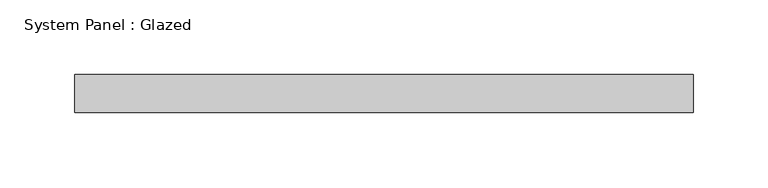
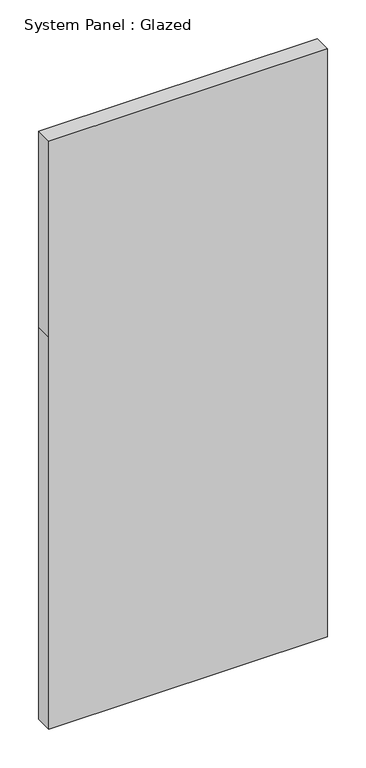
"""IFC4 building model written with IfcOpenShell, lengths in millimetres: plate geometry, System Panel : Glazed."""

from ifc_helpers import new_model, si_unit, frame, origin, place, context, project, spatial, polyline, outline, extrude, source, transform, mapped, element, save


def system_panel_glazed_1c8147a1(model_context):
    return source(origin(), model_context, "Body", "SweptSolid", [
        extrude(outline(polyline([(0.0, -206.375), (0.0, 206.375), (613.8333333, 206.375), (920.75, 206.375), (920.75, -206.375), (613.8333333, -206.375), (0.0, -206.375)])), frame((0.0, 19.05, 0.0), z_axis=(0.0, 1.0, 0.0), x_axis=(0.0, 0.0, 1.0)), (0.0, 0.0, 1.0), 25.4),
    ])


if __name__ == "__main__":
    model = new_model("IFC4")
    model_context = context("Model", 3, world=origin())
    ifc_project = project(units=[si_unit("LENGTHUNIT", "METRE", prefix="MILLI")], contexts=[model_context])
    site = spatial("IfcSite", under=ifc_project)
    building = spatial("IfcBuilding", under=site)
    placement = place(None, origin())
    system_panel_glazed_shape = system_panel_glazed_1c8147a1(model_context)
    element("IfcPlate", 1, ObjectType="System Panel : Glazed", at=placement, inside=building, context=model_context, shape_type="MappedRepresentation", body=[
        mapped(system_panel_glazed_shape, transform((0.0, 0.0, 0.0), x_axis=(1.0, 0.0, 0.0), y_axis=(0.0, 1.0, 0.0), z_axis=(0.0, 0.0, 1.0))),
    ])
    save(model, "model.ifc")

# Revit data of these elements
# Type "System Panel : Glazed"
#   Construction Type Id = "GSP4R"
#   Analytic Construction = "1/8 in Pilkington single glazing"
#   Visual Light Transmittance = 0.9
#   Solar Heat Gain Coefficient = 0.86
#   Heat Transfer Coefficient (U) = 1.18115 BTU/(h·ft²·°F)
#   Define Thermal Properties by = 1
# Element 1 (IfcPlate, "System Panel : Glazed")
#   Materials on its faces: "Glass"
# Materials
#   "Glass": class "Glass", colour RGB 0 128 192, transparency 0.75, Description = "Soda Lime Glass", Cost = 0
